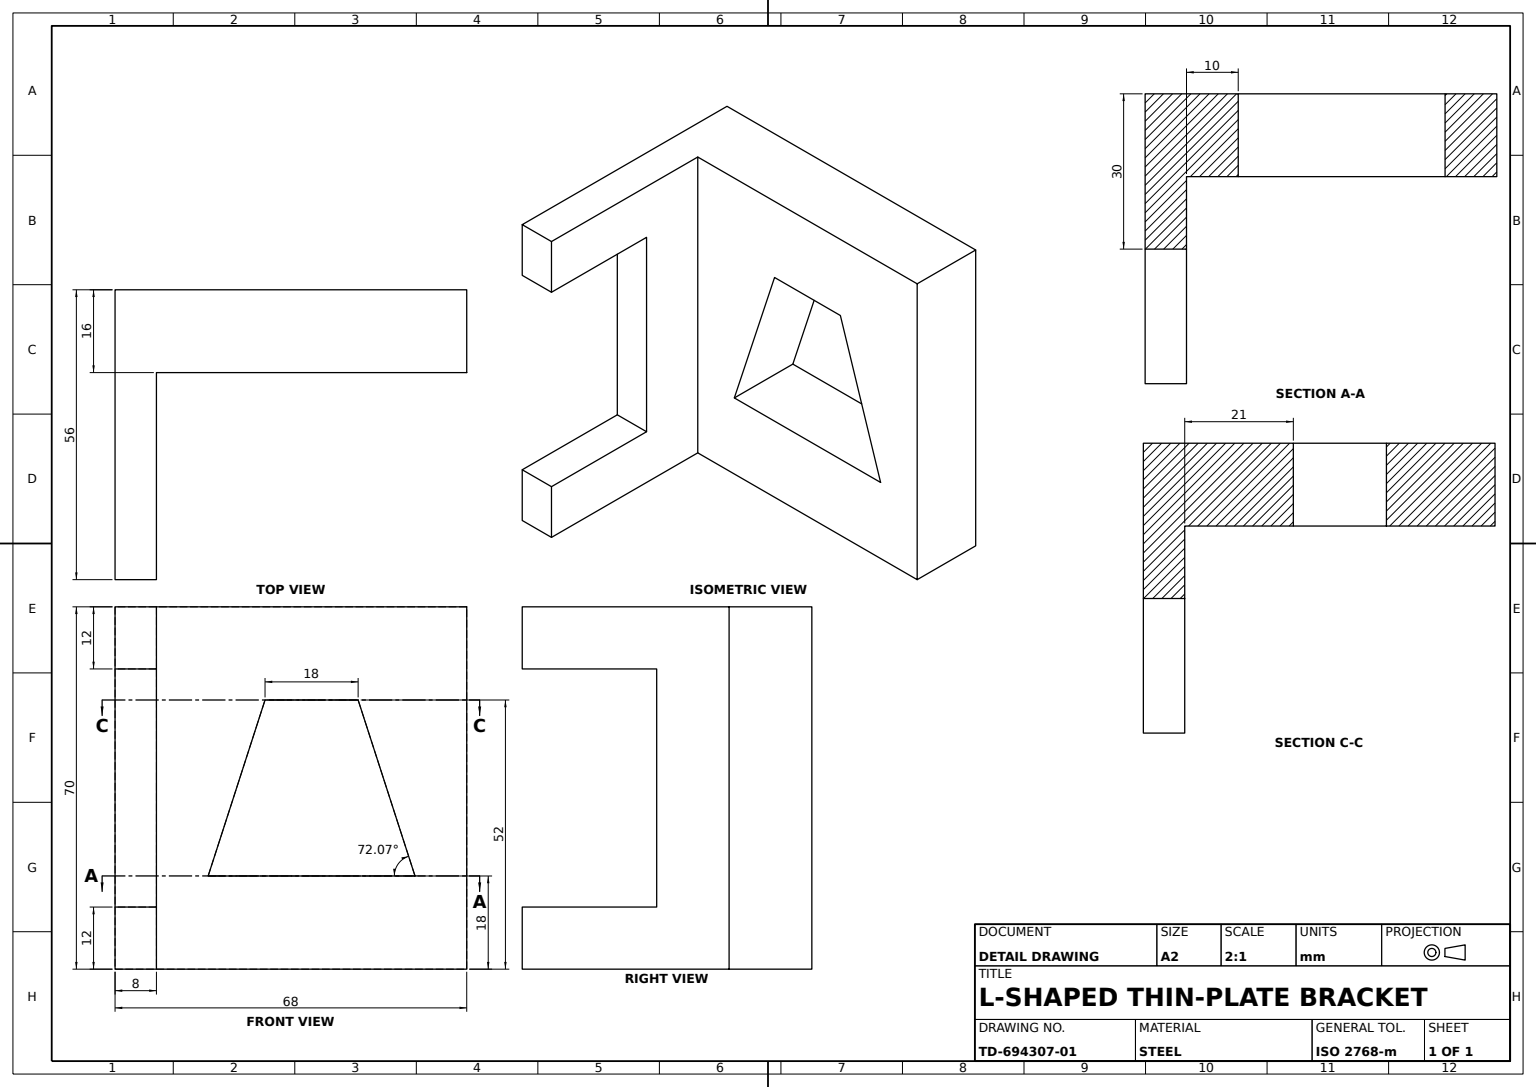
from build123d import *

# Parameters (mm, degrees)
BASE_PLATE_SKETCH_W     = 68
BASE_PLATE_SKETCH_H     = 70
BASE_PLATE_16MM_DEPTH   = 16
C_SIDE_FLANGE_8MM_DEPTH = 8
WINDOW_CUT_OUT_DEPTH    = 18


with BuildPart() as part:
    # Base Plate Sketch → Base Plate 16mm (new body)
    with BuildSketch(Plane.XY):
        with Locations((34, 35)):
            Rectangle(BASE_PLATE_SKETCH_W, BASE_PLATE_SKETCH_H)
    extrude(amount=BASE_PLATE_16MM_DEPTH)

    # Side Flange Sketch → C Side Flange 8mm (add)
    with BuildSketch(Plane.ZY):
        Polygon((16, 70), (56, 70), (56, 58), (30, 58), (30, 12), (56, 12), (56, 0), (16, 0), (0, 0), (0, 70), align=None)
    extrude(amount=-C_SIDE_FLANGE_8MM_DEPTH)

    # Window Sketch → Window Cut-Out (cut)
    with BuildSketch(Plane.XY.offset(16)):
        Polygon((58, 18), (18, 18), (29, 52), (38, 52), (47, 52), align=None)
    extrude(amount=-WINDOW_CUT_OUT_DEPTH, mode=Mode.SUBTRACT)


solid = part.part
